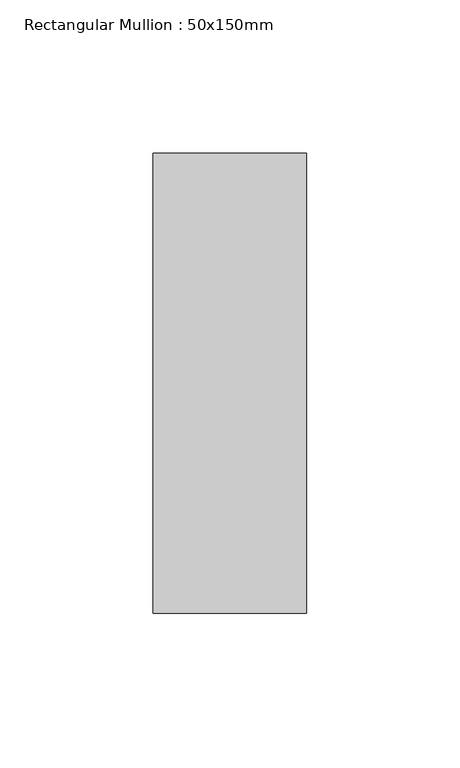
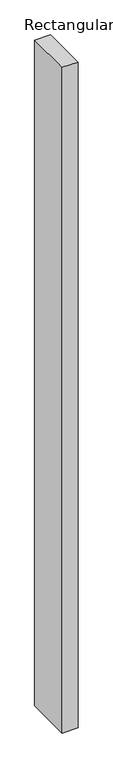
"""IFC4 building model written with IfcOpenShell, lengths in millimetres: member geometry, Rectangular Mullion : 50x150mm."""

from ifc_helpers import new_model, si_unit, frame, origin, place, context, project, spatial, polyline, outline, extrude, source, transform, mapped, element, save


def rectangular_mullion_50x150mm_8753fc4c(model_context):
    return source(origin(), model_context, "Body", "SweptSolid", [
        extrude(outline(polyline([(0.0, 75.0), (0.0, -75.0), (-50.0, -75.0), (-50.0, 75.0), (0.0, 75.0)])), frame((0.0, 0.0, -2219.3021954), z_axis=(0.0, 0.0, 1.0), x_axis=(1.0, 0.0, 0.0)), (0.0, 0.0, 1.0), 2219.3021954),
    ])


if __name__ == "__main__":
    model = new_model("IFC4")
    model_context = context("Model", 3, world=origin())
    ifc_project = project(units=[si_unit("LENGTHUNIT", "METRE", prefix="MILLI")], contexts=[model_context])
    site = spatial("IfcSite", under=ifc_project)
    building = spatial("IfcBuilding", under=site)
    placement = place(None, origin())
    rectangular_mullion_50x150mm_shape = rectangular_mullion_50x150mm_8753fc4c(model_context)
    element("IfcMember", 1, ObjectType="Rectangular Mullion : 50x150mm", at=placement, inside=building, context=model_context, shape_type="MappedRepresentation", body=[
        mapped(rectangular_mullion_50x150mm_shape, transform((0.0, 0.0, 0.0), x_axis=(1.0, 0.0, 0.0), y_axis=(0.0, 1.0, 0.0), z_axis=(0.0, 0.0, 1.0))),
    ])
    save(model, "model.ifc")

# Revit data of these elements
# Type "Rectangular Mullion : 50x150mm"
#   Keynote = "H11"
#   built-in parameter 1007304 = 0.492126 (stored number, unit not read)
#   built-in parameter 1007301 = 0.082021 (stored number, unit not read)
#   built-in parameter 1007300 = 0.082021 (stored number, unit not read)
# Element 1 (IfcMember, "Rectangular Mullion : 50x150mm")
#   Materials on its faces: "Aluminium"
# Materials
#   "Aluminium": class "Metal", colour RGB 247 247 247, transparency 0, Description = "Aluminium 6061", Cost = 0
